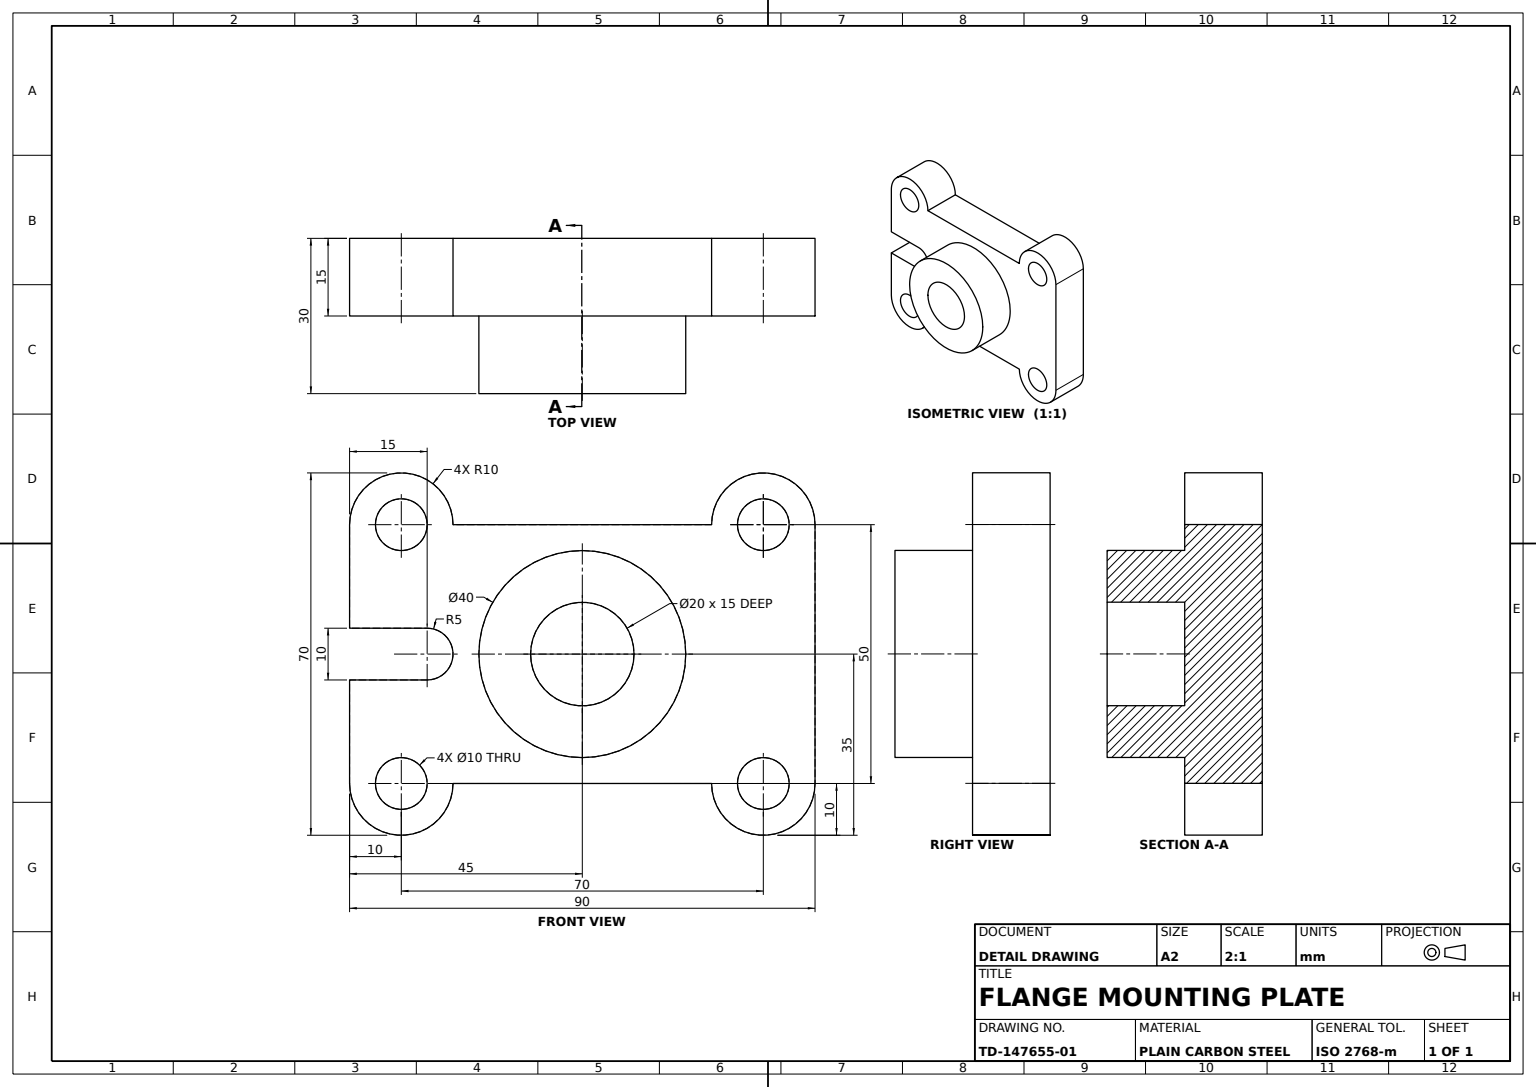
SolidWorks part; units mm, degrees
material "Plain Carbon Steel"
ref_plane "Front Plane" through (0, 0, 0) normal (0, 0, 1) x (1, 0, 0)
ref_plane "Top Plane" through (0, 0, 0) normal (0, 1, 0) x (1, 0, 0)
ref_plane "Right Plane" through (0, 0, 0) normal (1, 0, 0) x (0, 0, -1)
sketch "Flange Plate Profile Sketch" plane through (0, 0, 0) normal (0, 0, 1) x (1, 0, 0)
  line L0 (10, 0) -> (60, 0)
  line L2 (60, -50) -> (10, -50)
  line L4 (80, 0) -> (80, -50)
  line L5 (-10, 0) -> (-10, -20)
  line L7 (-10, -20) -> (5, -20)
  line L9 (5, -30) -> (-10, -30)
  line L10 (-10, -30) -> (-10, -50)
  arc A0 (10, 0) -> (-10, 0) centre (0, 0) ccw
  arc A1 (80, 0) -> (60, 0) centre (70, 0) ccw
  arc A2 (60, -50) -> (80, -50) centre (70, -50) ccw
  arc A3 (-10, -50) -> (10, -50) centre (0, -50) ccw
  arc A4 (5, -30) -> (5, -20) centre (5, -25) ccw
  point P6 (70, 10)
  point P19 (70, -60)
  point P20 (0, -60)
  point P21 (0, 10)
  point P22 (10, -25)
  dimension "D1" = 20
  dimension "D2" = 20
  dimension "D3" = 20
  dimension "D4" = 20
  dimension "D5" = 10
  dimension "D8" = 10
  dimension "D9" = 10
  dimension "D10" = 10
  dimension "D11" = 5
  dimension "D6" = 50
  dimension "D7" = 50
  dimension "D12" = 70
  dimension "D13" = 20
  dimension "D14" = 15
  dimension "D15" = 70
  dimension "D16" = 20
  dimension "D17" = 50
  dimension "D18" = 35
  dimension "D19" = 10
extrude "Flange Plate" add sketch "Flange Plate Profile Sketch" along normal blind 15
sketch "Side Notch Sketch" plane through (0, 0, 15) normal (0, 0, 1) x (1, 0, 0)
  circle A0 centre (0, 0) radius 5
  circle A1 centre (70, 0) radius 5
  circle A2 centre (70, -50) radius 5
  circle A3 centre (0, -50) radius 5
  dimension "D1" = 10
  dimension "D2" = 10
  dimension "D3" = 10
  dimension "D4" = 10
  dimension "D5" = 10
extrude "Side Notch 10x10" cut sketch "Side Notch Sketch" against normal blind 15
sketch "Hub Boss Sketch" plane through (0, 0, 15) normal (0, 0, 1) x (1, 0, 0)
  line L0 (80, -50) -> (80, 0) construction
  line L1 (10, -50) -> (60, -50) construction
  circle A0 centre (35, -25) radius 20
  dimension "D1" = 40
  dimension "D2" = 40
  dimension "D3" = 45
  dimension "D4" = 25
extrude "Hub Boss Ø40" add sketch "Hub Boss Sketch" along normal blind 15
sketch "Bore Sketch" plane through (0, 0, 30) normal (0, 0, 1) x (1, 0, 0)
  circle A0 centre (35, -25) radius 10
  dimension "D1" = 20
  dimension "D2" = 20
extrude "Bore Ø20" cut sketch "Bore Sketch" against normal blind 15
